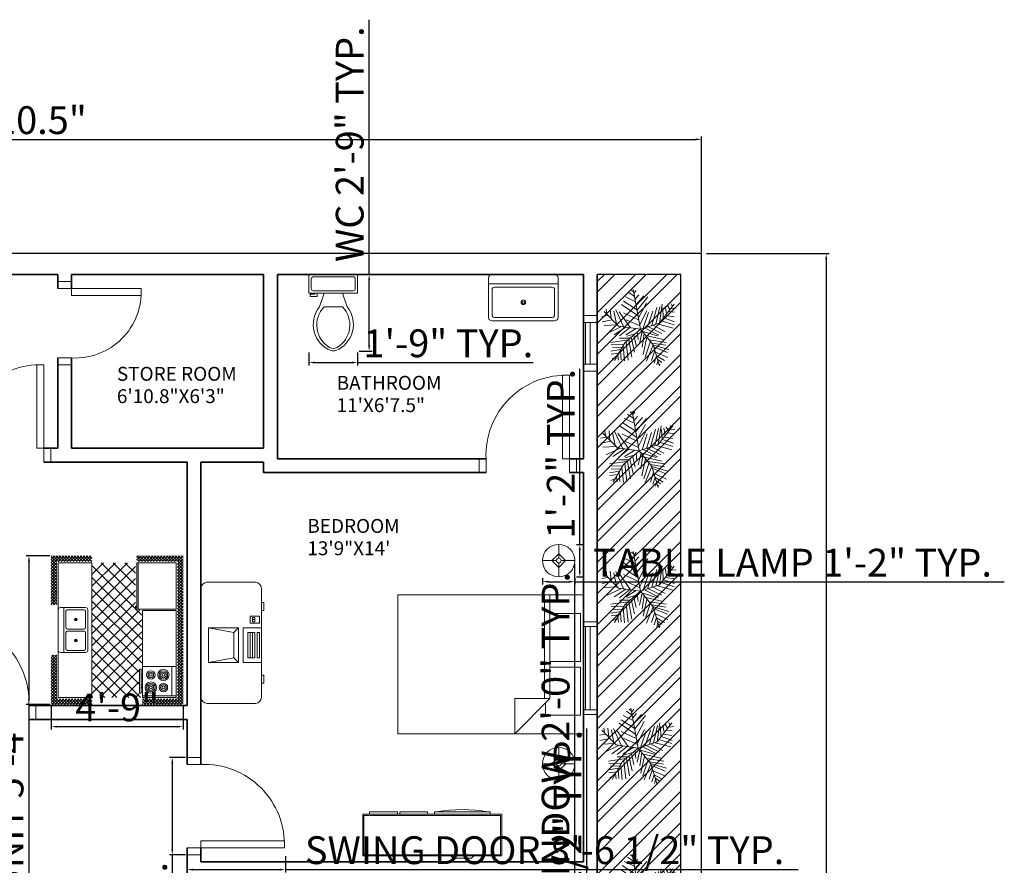
# Model space of a CAD drawing. Units: inches. Extents: x 2297 to 3143, y 440 to 1351.
# Tile 6 of 6: x 2697 to 3122, y 944 to 1309. Entities that reach past the tile are written whole.
import ezdxf

# ---------------------------------------------------------------- set-up
doc = ezdxf.new("R2010")
doc.units = ezdxf.units.IN
for name, color, linetype, lineweight in [('A-ANNO-DIMS', 2, 'Continuous', 18), ('A-AREA-IDEN', 7, 'Continuous', 18), ('A-DOOR', 4, 'Continuous', 20), ('A-EQPM', 8, 'Continuous', 18), ('A-FLOR-FIXT', 9, 'Continuous', 18), ('A-FURN', 8, 'Continuous', 18), ('A-GLAZ', 4, 'Continuous', 18), ('A-WALL', 7, 'Continuous', 35), ('C-PROP', 7, 'Continuous', 25), ('C-SITE-PATT', 252, 'Continuous', 13), ('E-LITE', 9, 'Continuous', 13), ('L-PLNT', 3, 'Continuous', 13)]:
    doc.layers.add(name, color=color, linetype=linetype, lineweight=lineweight)
doc.styles.get("Standard").update_dxf_attribs({"font": 'arial.ttf'})
doc.dimstyles.new('ISO-25', dxfattribs={"dimtxt": 12, "dimasz": 2.5, "dimexe": 1.25, "dimexo": 0.625, "dimtad": 1, "dimdec": 1, "dimlunit": 3, "dimtxsty": 'Standard', "dimcen": 2.5, "dimadec": 0, "dimazin": 0, "dimtfac": 1, "dimtdec": 1, "dimtmove": 0, "dimatfit": 3, "dimfxl": 1, "dimarcsym": 0})

# ---------------------------------------------------------------- blocks, each defined once
blk = doc.blocks.new('Kitchen Layout - 7 x 8 ft')
for p, q in [((-5, 81.32), (2.68, 89)), ((-5, 83.44), (0.56, 89)), ((-5, 85.56), (-1.56, 89)), ((-5, 87.68), (-3.68, 89)), ((-1, 84.97), (-5, 88.97)), ((-1, 82.85), (-5, 86.85)), ((-1, 80.73), (-5, 84.73)), ((1.09, 85), (-2.91, 89)), ((3.21, 85), (-0.79, 89)), ((0.81, 85), (4.81, 89)), ((5.34, 85), (1.34, 89)), ((2.93, 85), (6.93, 89)), ((7.46, 85), (3.46, 89)), ((5.05, 85), (9.05, 89)), ((9.58, 85), (5.58, 89)), ((7.17, 85), (11.17, 89)), ((11.7, 85), (7.7, 89)), ((9.29, 85), (13.29, 89)), ((13.82, 85), (9.82, 89)), ((11.41, 85), (15.41, 89)), ((15.94, 85), (11.94, 89)), ((13.53, 85), (17.53, 89)), ((18.06, 85), (14.06, 89)), ((15.65, 85), (19.65, 89)), ((20.18, 85), (16.18, 89)), ((17.78, 85), (21.78, 89)), ((22.31, 85), (18.31, 89)), ((19.9, 85), (23.9, 89)), ((24.43, 85), (20.43, 89)), ((22.02, 85), (26.02, 89)), ((26.55, 85), (22.55, 89)), ((24.14, 85), (28.14, 89)), ((28.67, 85), (24.67, 89)), ((26.26, 85), (30.26, 89)), ((30.79, 85), (26.79, 89)), ((28.38, 85), (32.38, 89)), ((32.91, 85), (28.91, 89)), ((30.5, 85), (34.5, 89)), ((35.03, 85), (31.03, 89)), ((32.63, 85), (36.63, 89)), ((37.16, 85), (33.16, 89)), ((34.75, 85), (38.75, 89)), ((39.28, 85), (35.28, 89)), ((36.87, 85), (40.87, 89)), ((41.4, 85), (37.4, 89)), ((38.99, 85), (42.99, 89)), ((43.52, 85), (39.52, 89)), ((41.11, 85), (45.11, 89)), ((45.64, 85), (41.64, 89)), ((43.23, 85), (47.23, 89)), ((47.76, 85), (43.76, 89)), ((45.35, 85), (49.35, 89)), ((49.88, 85), (45.88, 89)), ((47.47, 85), (51.47, 89)), ((52, 85), (48, 89)), ((49.6, 85), (53.6, 89)), ((54.13, 85), (50.13, 89)), ((51.72, 85), (55.72, 89)), ((56.25, 85), (52.25, 89)), ((53.84, 85), (57.84, 89)), ((58.37, 85), (54.37, 89)), ((55.96, 85), (59.96, 89)), ((60.49, 85), (56.49, 89)), ((58.08, 85), (62.08, 89)), ((62.61, 85), (58.61, 89)), ((60.2, 85), (64.2, 89)), ((64.73, 85), (60.73, 89)), ((62.32, 85), (66.32, 89)), ((66.85, 85), (62.85, 89)), ((64.45, 85), (68.45, 89)), ((68.97, 85), (64.97, 89)), ((66.57, 85), (70.57, 89)), ((71.1, 85), (67.1, 89)), ((68.69, 85), (72.69, 89)), ((73.22, 85), (69.22, 89)), ((70.81, 85), (74.81, 89)), ((75.34, 85), (71.34, 89)), ((72.93, 85), (76.93, 89)), ((77.46, 85), (73.46, 89)), ((75.05, 85), (79.05, 89)), ((79.58, 85), (75.58, 89)), ((77.17, 85), (81.17, 89)), ((81.7, 85), (77.7, 89)), ((79.29, 85), (83.29, 89)), ((83.82, 85), (79.82, 89)), ((81.42, 85), (85.42, 89)), ((85.95, 85), (81.95, 89)), ((83.54, 85), (87.54, 89)), ((88.07, 85), (84.07, 89)), ((85.66, 85), (89.66, 89)), ((90.19, 85), (86.19, 89)), ((87.78, 85), (91.78, 89)), ((92.31, 85), (88.31, 89)), ((89.9, 85), (93.9, 89)), ((94.43, 85), (90.43, 89)), ((92.02, 85), (96.02, 89)), ((96.55, 85), (92.55, 89)), ((94.14, 85), (98.14, 89)), ((101, 82.67), (94.67, 89)), ((96.27, 85), (100.27, 89)), ((101, 84.79), (96.79, 89)), ((97, 83.61), (101, 87.61)), ((97, 81.49), (101, 85.49)), ((101, 80.55), (97, 84.55)), ((101, 86.92), (98.92, 89)), ((-5, 79.19), (-1, 83.19)), ((-1, 78.61), (-5, 82.61)), ((-5, 77.07), (-1, 81.07)), ((-1, 76.49), (-5, 80.49)), ((-5, 74.95), (-1, 78.95)), ((-1, 74.36), (-5, 78.36)), ((34, 84), (96, 84)), ((34, 60), (34, 84)), ((74, 81), (95, 81)), ((96, 84), (96, 60)), ((97, 79.37), (101, 83.37)), ((101, 78.43), (97, 82.43)), ((97, 77.25), (101, 81.25)), ((101, 76.31), (97, 80.31)), ((97, 75.13), (101, 79.13)), ((101, 74.19), (97, 78.19)), ((-5, 72.83), (-1, 76.83)), ((-1, 72.24), (-5, 76.24)), ((-5, 70.71), (-1, 74.71)), ((-1, 70.12), (-5, 74.12)), ((-5, 68.59), (-1, 72.59)), ((-1, 68), (-5, 72)), ((-5, 66.47), (-1, 70.47)), ((97, 73.01), (101, 77.01)), ((101, 72.07), (97, 76.07)), ((97, 70.89), (101, 74.89)), ((101, 69.95), (97, 73.95)), ((97, 68.76), (101, 72.76)), ((101, 67.82), (97, 71.82)), ((97, 66.64), (101, 70.64)), ((-1, 65.88), (-5, 69.88)), ((-5, 64.35), (-1, 68.35)), ((-1, 63.76), (-5, 67.76)), ((-5, 62.22), (-1, 66.22)), ((-1, 61.64), (-5, 65.64)), ((-5, 60.1), (-1, 64.1)), ((-1, 59.52), (-5, 63.52)), ((101, 65.7), (97, 69.7)), ((97, 64.52), (101, 68.52)), ((101, 63.58), (97, 67.58)), ((97, 62.4), (101, 66.4)), ((101, 61.46), (97, 65.46)), ((97, 60.28), (101, 64.28)), ((100.34, 60), (97, 63.34)), ((-5, 57.98), (-1, 61.98)), ((-1, 57.39), (-5, 61.39)), ((-1.73, 56), (-5, 59.27)), ((-3.85, 56), (-5, 57.15)), ((-4.86, 56), (-1, 59.86)), ((-2.74, 56), (-1, 57.74)), ((0, 57), (33, 57)), ((10.4, 24), (45.9, 59.5)), ((18.88, 24), (54.38, 59.5)), ((27.37, 24), (62.87, 59.5)), ((33.03, 55.11), (37.41, 59.5)), ((67.71, 24), (33.68, 58.04)), ((96, 60), (34, 60)), ((35.85, 24), (71.35, 59.5)), ((76.2, 24), (40.7, 59.5)), ((44.34, 24), (77.84, 57.5)), ((84.68, 24), (49.18, 59.5)), ((52.82, 24), (86.32, 57.5)), ((93.17, 24), (57.67, 59.5)), ((61.31, 24), (96, 58.69)), ((96, 29.65), (66.15, 59.5)), ((96, 38.14), (76.64, 57.5)), ((80, 60), (80, 59)), ((82, 59), (82, 60)), ((96, 46.63), (85.13, 57.5)), ((87, 59), (87, 60)), ((89, 60), (89, 59)), ((96, 55.11), (93.57, 57.54)), ((98.22, 60), (97, 61.22)), ((98.84, 60), (101, 62.16)), ((100.96, 60), (101, 60.04)), ((0, 30.57), (24.43, 55)), ((0, 39.06), (15.94, 55)), ((0, 47.54), (7.46, 55)), ((25.29, 24), (0, 49.29)), ((1.91, 24), (32.91, 55)), ((33.77, 24), (2.77, 55)), ((42.26, 24), (11.26, 55)), ((50.74, 24), (19.74, 55)), ((59.23, 24), (28.23, 55)), ((31, 55), (31, 56)), ((32, 55), (31, 55)), ((32, 56), (32, 55)), ((69.79, 24), (96, 50.21)), ((16.8, 24), (0, 40.8)), ((78.28, 24), (96, 41.72)), ((8.32, 24), (0, 32.32)), ((86.76, 24), (96, 33.24)), ((-5, 21.92), (-2.92, 24)), ((-5, 19.8), (-1, 23.8)), ((-1, 19.21), (-5, 23.21)), ((-5, 17.68), (-1, 21.68)), ((-1, 17.09), (-5, 21.09)), ((-1, 21.33), (-3.67, 24)), ((-1, 23.45), (-1.55, 24)), ((0, 24), (96, 24)), ((0, 0), (0, 24)), ((95.25, 24), (96, 24.75)), ((96, 24), (96, 0)), ((97, 22.1), (98.9, 24)), ((97, 19.97), (101, 23.97)), ((101, 19.03), (97, 23.03)), ((97, 17.85), (101, 21.85)), ((101, 21.16), (98.16, 24)), ((101, 23.28), (100.28, 24)), ((-5, 15.55), (-1, 19.55)), ((-1, 14.97), (-5, 18.97)), ((-5, 13.43), (-1, 17.43)), ((-1, 12.85), (-5, 16.85)), ((-5, 11.31), (-1, 15.31)), ((-1, 10.73), (-5, 14.73)), ((47.25, 6.5), (47.25, 18.5)), ((48.75, 18.5), (48.75, 6.5)), ((101, 16.91), (97, 20.91)), ((97, 15.73), (101, 19.73)), ((101, 14.79), (97, 18.79)), ((97, 13.61), (101, 17.61)), ((101, 12.67), (97, 16.67)), ((97, 11.49), (101, 15.49)), ((101, 10.55), (97, 14.55)), ((-5, 9.19), (-1, 13.19)), ((-1, 8.6), (-5, 12.6)), ((-5, 7.07), (-1, 11.07)), ((-1, 6.48), (-5, 10.48)), ((-5, 4.95), (-1, 8.95)), ((-1, 4.36), (-5, 8.36)), ((97, 9.37), (101, 13.37)), ((101, 8.43), (97, 12.43)), ((97, 7.25), (101, 11.25)), ((101, 6.31), (97, 10.31)), ((97, 5.12), (101, 9.12)), ((101, 4.18), (97, 8.18)), ((-5, 2.83), (-1, 6.83)), ((-1, 2.24), (-5, 6.24)), ((-5, 0.71), (-1, 4.71)), ((-1, 0.12), (-5, 4.12)), ((-5, -1.42), (-1, 2.58)), ((2, -5), (-5, 2)), ((-5, -3.54), (-1, 0.46)), ((96, 0), (0, 0)), ((64, 4), (32, 4)), ((93.24, -5), (101, 2.76)), ((95.36, -5), (101, 0.64)), ((97, 3), (101, 7)), ((101, 2.06), (97, 6.06)), ((97, 0.88), (101, 4.88)), ((101, -0.06), (97, 3.94)), ((101, -2.18), (97, 1.82)), ((-0.12, -5), (-5, -0.12)), ((-2.25, -5), (-5, -2.25)), ((-4.37, -5), (-5, -4.37)), ((-4.34, -5), (-0.34, -1)), ((-2.22, -5), (1.78, -1)), ((-0.1, -5), (3.9, -1)), ((4.12, -5), (0.12, -1)), ((2.02, -5), (6.02, -1)), ((6.24, -5), (2.24, -1)), ((4.14, -5), (8.14, -1)), ((8.36, -5), (4.36, -1)), ((6.27, -5), (10.27, -1)), ((10.48, -5), (6.48, -1)), ((8.39, -5), (12.39, -1)), ((12.6, -5), (8.6, -1)), ((10.51, -5), (14.51, -1)), ((14.73, -5), (10.73, -1)), ((12.63, -5), (16.63, -1)), ((16.85, -5), (12.85, -1)), ((14.75, -5), (18.75, -1)), ((18.97, -5), (14.97, -1)), ((16.87, -5), (20.87, -1)), ((21.09, -5), (17.09, -1)), ((18.99, -5), (22.99, -1)), ((23.21, -5), (19.21, -1)), ((21.11, -5), (25.11, -1)), ((25.33, -5), (21.33, -1)), ((23.24, -5), (27.24, -1)), ((27.45, -5), (23.45, -1)), ((25.36, -5), (29.36, -1)), ((29.57, -5), (25.57, -1)), ((27.48, -5), (30, -2.48)), ((30, -3.3), (27.7, -1)), ((29.6, -5), (30, -4.6)), ((30, -1.18), (29.82, -1)), ((66, -2.54), (67.54, -1)), ((66, -4.66), (69.66, -1)), ((69.88, -5), (66, -1.12)), ((67.76, -5), (66, -3.24)), ((67.78, -5), (71.78, -1)), ((72, -5), (68, -1)), ((69.9, -5), (73.9, -1)), ((74.12, -5), (70.12, -1)), ((72.03, -5), (76.03, -1)), ((76.24, -5), (72.24, -1)), ((74.15, -5), (78.15, -1)), ((78.36, -5), (74.36, -1)), ((76.27, -5), (80.27, -1)), ((80.49, -5), (76.49, -1)), ((78.39, -5), (82.39, -1)), ((82.61, -5), (78.61, -1)), ((80.51, -5), (84.51, -1)), ((84.73, -5), (80.73, -1)), ((82.63, -5), (86.63, -1)), ((86.85, -5), (82.85, -1)), ((84.75, -5), (88.75, -1)), ((88.97, -5), (84.97, -1)), ((86.88, -5), (90.88, -1)), ((91.09, -5), (87.09, -1)), ((89, -5), (93, -1)), ((93.21, -5), (89.21, -1)), ((91.12, -5), (95.12, -1)), ((95.34, -5), (91.34, -1)), ((97.46, -5), (93.46, -1)), ((99.58, -5), (95.58, -1)), ((101, -4.3), (97, -0.3)), ((97.48, -5), (101, -1.48)), ((99.6, -5), (101, -3.6))]:
    blk.add_line(p, q)
for points in [[(0, 56), (0, 84), (33, 84), (33, 56)], [(74, 60), (74, 84), (95, 84), (95, 60)], [(76, 58), (76, 59), (93, 59), (93, 58)]]:
    blk.add_lwpolyline(points, close=True)
for points in [[(32, 1.5), (32, 19.5)], [(33.5, 21), (62.5, 21)], [(33.5, 6.5), (33.5, 18.5)], [(34.5, 19.5), (46.25, 19.5)], [(49.75, 19.5), (61.5, 19.5)], [(62.5, 18.5), (62.5, 6.5)], [(64, 19.5), (64, 1.5)], [(62.5, 0), (33.5, 0)], [(46.25, 5.5), (34.5, 5.5)], [(61.5, 5.5), (49.75, 5.5)]]:
    blk.add_lwpolyline(points)
for centre, radius in [((80, 75), 4), ((80, 75), 3), ((89, 75), 3), ((80, 75), 2), ((80, 75), 1), ((89, 75), 2), ((89, 75), 1), ((80, 66), 3), ((80, 66), 2), ((80, 66), 1), ((89, 66), 4), ((89, 66), 3), ((89, 66), 2), ((89, 66), 1), ((40.5, 12.5), 1), ((40.5, 12.5), 0.5), ((55.5, 12.5), 1), ((55.5, 12.5), 0.5)]:
    blk.add_circle(centre, radius)
for centre, radius, start, end in [((33.5, 19.5), 1.5, 90, 180), ((34.5, 18.5), 1, 90, 180), ((46.25, 18.5), 1, 0, 90), ((49.75, 18.5), 1, 90, 180), ((61.5, 18.5), 1, 0, 90), ((62.5, 19.5), 1.5, 0, 90), ((33.5, 1.5), 1.5, 180, 270), ((34.5, 6.5), 1, 180, 270), ((46.25, 6.5), 1, 270, 0), ((49.75, 6.5), 1, 180, 270), ((61.5, 6.5), 1, 270, 0), ((62.5, 1.5), 1.5, 270, 0)]:
    blk.add_arc(centre, radius, start, end)
blk = doc.blocks.new('Bed - Queen')
for p, q in [((0, -80.00003), (0, 0)), ((0, 0), (59.99999, 0)), ((59.99999, 0), (59.99999, -80.00003)), ((7.99999, -1.2), (28.79998, -1.2)), ((7.99999, -14.4), (7.99999, -1.2)), ((28.79998, -1.2), (28.79998, -14.4)), ((31.19999, -1.2), (51.99999, -1.2)), ((31.19999, -14.4), (31.19999, -1.2)), ((51.99999, -1.2), (51.99999, -16.4)), ((0, -14.4), (44.8, -14.4)), ((44.8, -16.8), (0, -16.8)), ((59.99999, -29.6), (44.8, -14.4)), ((44.8, -14.4), (44.8, -29.6)), ((51.99999, -16.4), (46.79936, -16.4)), ((44.8, -29.6), (59.99999, -29.6)), ((59.99999, -80.00003), (0, -80.00003))]:
    blk.add_line(p, q)
blk = doc.blocks.new('Sink-single - 30 in top')
blk.add_line((-15, -3.999996), (15, -3.999996))
for points in [[(-13.5, 0), (13.5, 0)], [(-15, -18.499996), (-15, -1.5)], [(15, -1.5), (15, -18.499996)], [(-13.5, -17.499996), (-13.5, -6.499996)], [(-12.5, -5.499996), (12.5, -5.499996)], [(13.5, -6.499996), (13.5, -17.499996)], [(13.5, -19.999996), (-13.5, -19.999996)], [(12.5, -18.499996), (-12.5, -18.499996)]]:
    blk.add_lwpolyline(points)
for radius in [1, 0.5]:
    blk.add_circle((0, -11.999996), radius)
for centre, radius, start, end in [((-13.5, -1.5), 1.5, 90, 180), ((13.5, -1.5), 1.5, 0, 90), ((-12.5, -6.499996), 1, 90, 180), ((12.5, -6.499996), 1, 0, 90), ((-13.5, -18.499996), 1.5, 180, 270), ((-12.5, -17.499996), 1, 180, 270), ((12.5, -17.499996), 1, 270, 0), ((13.5, -18.499996), 1.5, 270, 0)]:
    blk.add_arc(centre, radius, start, end)
blk = doc.blocks.new('Toilet - top')
for p, q in [((9.5, -6), (9.5, -2)), ((-8, -8.5), (-8, -8)), ((-7, -8), (-7, -9.5)), ((-4, -8), (-6, -14)), ((4, -8), (6, -14)), ((-10, -8.5), (-8, -8.5)), ((-10, -9.5), (-10, -8.5)), ((-7, -9.5), (-10, -9.5)), ((4, -14), (-4, -14))]:
    blk.add_line(p, q)
blk.add_lwpolyline([(10.5, -8), (10.5, 0), (-10.5, 0), (-10.5, -8)], close=True)
for points in [[(-9.5, -2), (-9.5, -6)], [(8.5, -1), (-8.5, -1)], [(-8.5, -7), (8.5, -7)]]:
    blk.add_lwpolyline(points)
for centre, radius, start, end in [((-8.62, -1.88), 0.884, 81.8699, 188.1301), ((8.62, -1.88), 0.884, 351.8699, 98.1301), ((-8.62, -6.12), 0.884, 171.8699, 278.1301), ((8.62, -6.12), 0.884, 261.8699, 8.1301), ((3.52, -21.58), 12.17, 141.4691, 247.9714), ((4.2, -21.82), 11.33, 136.3677, 238.9468), ((-3.52, -21.58), 12.17, 292.0284, 38.5307), ((-4.2, -21.82), 11.33, 301.053, 43.6321), ((0, -27.88), 4, 245.7318, 294.2682), ((0, -29), 4, 254.8605, 285.1395)]:
    blk.add_arc(centre, radius, start, end)
blk = doc.blocks.new('*U16')
for p, q in [((0, 0), (-10.5, 57)), ((-7.288, 39.707), (-21.778, 46.673)), ((-8.737, 47.138), (-17.069, 52.711)), ((-10.186, 53.64), (-13.084, 55.962)), ((-9.099, 51.782), (-6.563, 55.962)), ((-7.65, 43.423), (-2.578, 49.46)), ((-5.839, 35.992), (4.667, 48.067)), ((-5.114, 27.632), (10.463, 46.673)), ((-48.585, 21.131), (-49.309, 29.026)), ((-43.513, 28.561), (-42.427, 15.558)), ((-3.665, 19.273), (-27.574, 35.527)), ((-5.114, 28.097), (-24.676, 40.636)), ((-2.941, 16.486), (8.652, 37.85)), ((16.259, 5.805), (23.142, 31.348)), ((22.055, 7.198), (27.489, 32.277)), ((27, 9), (48, 36)), ((27.127, 9.056), (31.112, 35.992)), ((31.836, 30.883), (32.561, 16.486)), ((35.096, 32.741), (37.27, 22.524)), ((38.719, 34.134), (41.979, 28.561)), ((43.791, 29.954), (51.036, 30.883)), ((44.153, 36.456), (45.239, 32.741)), ((-47.498, 19.737), (-55.83, 18.344)), ((-31.5, 4.5), (-52.5, 25.5)), ((-38.442, 26.239), (-34.819, 7.663)), ((-35.544, 28.097), (-24.314, 3.947)), ((-14.533, 2.09), (-30.834, 25.31)), ((-24.314, 23.917), (-2.941, 13.7)), ((-1.129, 6.734), (9.014, 26.704)), ((3.942, 1.625), (11.187, 24.381)), ((10.101, 3.483), (17.708, 26.239)), ((33.285, 16.486), (48.862, 10.913)), ((36.183, 19.737), (48.137, 17.88)), ((40.53, 25.775), (48.862, 24.846)), ((-40.615, 13.7), (-55.105, 10.913)), ((-33.37, 6.269), (-52.207, 5.34)), ((-28.299, 3.483), (-47.86, -5.805)), ((-21.416, 3.018), (-38.079, -8.128)), ((0, 0), (-31.5, 4.5)), ((-15.982, 2.09), (-30.11, -9.521)), ((0, 0), (-22.5, -19.5)), ((-6.563, 1.161), (-21.416, -8.128)), ((-20.691, 13.7), (-1.129, 4.876)), ((0, 0), (27, 9)), ((0, 0), (18, -22.5)), ((6.478, 1.625), (26.04, -8.592)), ((11.187, 3.483), (30.749, -5.805)), ((18.07, 5.805), (35.096, -3.483)), ((24.229, 7.663), (46.688, 1.625)), ((29.662, 12.307), (48.137, 6.269)), ((-15.257, -12.772), (-30.11, -12.772)), ((-6.563, -5.805), (-19.967, -9.985)), ((-13.446, -11.378), (-8.737, -32.741)), ((-9.461, -8.592), (-6.201, -23.453)), ((-4.752, -3.483), (-3.665, -14.629)), ((2.493, -3.019), (-1.491, -20.202)), ((1.769, -2.555), (24.229, -9.521)), ((5.029, -6.27), (2.131, -25.775)), ((9.014, -11.378), (3.58, -35.992)), ((7.565, -9.056), (32.198, -14.629)), ((-17.431, -15.094), (-42.789, -18.809)), ((-24.314, -21.596), (-42.427, -22.06)), ((-26.849, -26.24), (-40.253, -25.775)), ((-22.5, -19.5), (-37.5, -45)), ((-25.038, -23.918), (-22.865, -45.281)), ((-20.691, -18.345), (-17.793, -44.352)), ((-17.069, -15.094), (-12.721, -40.172)), ((14.085, -16.951), (6.478, -40.172)), ((18.07, -22.524), (8.289, -45.745)), ((12.274, -15.094), (36.907, -18.809)), ((16.259, -19.738), (36.183, -22.989)), ((18, -22.5), (27, -52.5)), ((18.433, -22.524), (40.53, -29.026)), ((19.157, -25.311), (38.719, -33.206)), ((-28.299, -29.026), (-42.789, -31.348)), ((-30.834, -34.135), (-42.427, -35.528)), ((-34.457, -39.708), (-40.978, -42.494)), ((-32.646, -36.921), (-31.921, -44.352)), ((-29.023, -30.884), (-27.936, -43.887)), ((20.244, -30.419), (15.897, -44.816)), ((22.78, -37.85), (19.519, -48.532)), ((21.331, -32.741), (39.081, -40.636)), ((22.78, -38.314), (34.372, -44.816)), ((24.591, -45.745), (23.142, -50.854)), ((24.591, -43.423), (30.749, -47.603)), ((26.764, -49.925), (28.213, -50.854))]:
    blk.add_line(p, q)
blk = doc.blocks.new('*D17')
at = {"layer": 'A-ANNO-DIMS', "color": 0, "lineweight": -2, "transparency": 16777216}
for p, q in [((2393.19, 1208.26), (2393.19, 1258.2)), ((2991.69, 1208.26), (2991.69, 1258.2)), ((2395.69, 1256.95), (2989.19, 1256.95))]:
    blk.add_line(p, q, dxfattribs=at)
at = {"layer": 'A-ANNO-DIMS', "color": 0, "transparency": 16777216}
for points in [[(2395.69, 1257.36), (2395.69, 1256.53), (2393.19, 1256.95)], [(2989.19, 1257.36), (2989.19, 1256.53), (2991.69, 1256.95)]]:
    blk.add_solid(points, dxfattribs=at)
at = {"layer": 'Defpoints', "color": 0, "transparency": 16777216}
for p in [(2991.69, 1256.95), (2393.19, 1207.63), (2991.69, 1207.63)]:
    blk.add_point(p, dxfattribs=at)
at = {"layer": 'A-ANNO-DIMS', "color": 0, "transparency": 16777216, "insert": (2692.44, 1263.7), "char_height": 12, "attachment_point": 5}
blk.add_mtext('49\'-10.5"', dxfattribs=at)
blk = doc.blocks.new('*D18')
at = {"layer": 'A-ANNO-DIMS', "color": 0, "lineweight": -2, "transparency": 16777216}
for p, q in [((2993.8, 1207.63), (3046.74, 1207.63)), ((3045.49, 1205.13), (3045.49, 550.13)), ((2992.32, 547.63), (3046.74, 547.63))]:
    blk.add_line(p, q, dxfattribs=at)
at = {"layer": 'A-ANNO-DIMS', "color": 0, "transparency": 16777216}
for points in [[(3045.07, 1205.13), (3045.91, 1205.13), (3045.49, 1207.63)], [(3045.07, 550.13), (3045.91, 550.13), (3045.49, 547.63)]]:
    blk.add_solid(points, dxfattribs=at)
at = {"layer": 'Defpoints', "color": 0, "transparency": 16777216}
for p in [(2993.18, 1207.63), (2991.69, 547.63), (3045.49, 547.63)]:
    blk.add_point(p, dxfattribs=at)
at = {"layer": 'A-ANNO-DIMS', "color": 0, "transparency": 16777216, "insert": (3038.76, 877.63), "char_height": 12, "attachment_point": 5, "rotation": 90}
blk.add_mtext("55'", dxfattribs=at)
blk = doc.blocks.new('Lamp - Table')
for p, q in [((0, 7), (0, 1)), ((-1, 0), (-7, 0)), ((0, 3), (-3, 0)), ((-3, 0), (0, -3)), ((3, 0), (0, 3)), ((0, -3), (3, 0)), ((1, 0), (7, 0)), ((0, -1), (0, -7))]:
    blk.add_line(p, q)
for radius in [7, 1]:
    blk.add_circle((0, 0), radius)
blk = doc.blocks.new('Desk - 30 x 60 in.')
for p, q in [((-26.999995, 0), (26.999995, 0)), ((-29.999995, -27), (-29.999995, -3)), ((29.999995, -3), (29.999995, -27)), ((26.999995, -30), (-26.999995, -30)), ((-20.000005, -30), (-20.000005, -31)), ((-20.000005, -31), (-16.000005, -31)), ((-16.000005, -31), (-16.000005, -30)), ((15.999995, -31), (15.999995, -30)), ((19.999995, -31), (15.999995, -31)), ((19.999995, -30), (19.999995, -31))]:
    blk.add_line(p, q)
for centre, start, end in [((-26.499995, -3.5), 98.1301, 171.8699), ((26.499995, -3.5), 8.130102, 81.8699), ((-26.499995, -26.5), 188.1301, 261.8699), ((26.499995, -26.5), 278.1301, 351.8699)]:
    blk.add_arc(centre, 3.535534, start, end)
blk = doc.blocks.new('Computer Terminal')
for p, q in [((-10, 11.5), (5, 11.5)), ((-8, 0.5), (-10, 11.5)), ((-10, -1.5), (-10, 11.5)), ((5, 11.5), (3, 0.5)), ((5, 11.5), (5, -1.5)), ((-10, -1.5), (-8, 0.5)), ((3, 0.5), (-8, 0.5)), ((3, 0.5), (5, -1.5)), ((5, -1.5), (-10, -1.5)), ((-10, -11.5), (-10, -3.5)), ((-10, -3.5), (5, -3.5)), ((5, -3.5), (5, -11.5)), ((-8, -5.5), (-8, -8.5)), ((3, -5.5), (-8, -5.5)), ((3, -6.5), (-8, -6.5)), ((-8, -7.5), (3, -7.5)), ((3, -8.5), (3, -5.5)), ((10, -6.5), (7, -6.5)), ((7, -6.5), (7, -10.5)), ((9.5, -7.5), (7.5, -7.5)), ((7.5, -7.5), (7.5, -8.5)), ((8.5, -7.5), (8.5, -8.5)), ((9.5, -8.5), (9.5, -7.5)), ((10, -10.5), (10, -6.5)), ((5, -11.5), (-10, -11.5)), ((-8, -8.5), (3, -8.5)), ((-8, -9.5), (-8, -10.5)), ((3, -9.5), (-8, -9.5)), ((-8, -10.5), (3, -10.5)), ((3, -10.5), (3, -9.5)), ((7, -10.5), (10, -10.5)), ((7.5, -8.5), (9.5, -8.5))]:
    blk.add_line(p, q)
blk = doc.blocks.new('Entertainment Center')
for p, q in [((-4, 0), (-5, -1)), ((4, 0), (-4, 0)), ((5, -1), (4, 0)), ((-17, -19), (-17, -1)), ((-17, -1), (43, -1)), ((-16.5, -18.5), (-16.5, -1.5)), ((-16.5, -1.5), (42.5, -1.5)), ((42.5, -1.5), (42.5, -18.5)), ((43, -1), (43, -19)), ((43, -19), (-17, -19)), ((42.5, -18.5), (-16.5, -18.5)), ((-12, -20), (-12, -19)), ((12, -20), (-12, -20)), ((12, -19), (12, -20)), ((15, -20), (15, -19)), ((27, -20), (15, -20)), ((27, -19), (27, -20)), ((28, -20), (28, -19)), ((40, -20), (28, -20)), ((40, -19), (40, -20))]:
    blk.add_line(p, q)
blk.add_arc((0, 40), 61, 259.6111, 280.3889)
blk = doc.blocks.new('DOOR-36IN-6IN-JAMB')
for p, q in [((0, 6), (0, 0)), ((3, 6), (3, 0)), ((39, 6), (39, 0)), ((42, 6), (42, 0))]:
    blk.add_line(p, q)
blk.add_lwpolyline([(39, 6), (36, 6), (36, 42), (39, 42)], close=True)
blk.add_arc((37.5, 7.5), 34.53, 87.5104, 182.4896)
blk = doc.blocks.new('DOOR-30IN-LEAF')
blk.add_lwpolyline([(30, 0), (27, 0), (27, 30), (30, 30)], close=True)
blk.add_arc((28.5, 1.5), 28.54, 86.9872, 183.0128)
blk = doc.blocks.new('WIN-36IN-6IN-WALL')
for p, q in [((6, 40), (0, 40)), ((6, 38), (0, 38)), ((3, 38), (3, 2)), ((5, 38), (5, 2)), ((0, 2), (6, 2)), ((0, 0), (6, 0))]:
    blk.add_line(p, q)
blk = doc.blocks.new('WIN-18IN-6IN-WALL')
for p, q in [((6, 24), (0, 24)), ((6, 21), (0, 21)), ((1, 3), (1, 21)), ((3, 3), (3, 21)), ((0, 3), (6, 3)), ((0, 0), (6, 0))]:
    blk.add_line(p, q)
blk = doc.blocks.new('*D27')
at = {"layer": 'A-ANNO-DIMS', "color": 0, "lineweight": -2, "transparency": 16777216}
for p, q in [((2923.06, 1067.52), (2923.06, 1064.79)), ((2937.06, 1067.52), (2937.06, 1064.79)), ((2925.56, 1066.04), (2934.56, 1066.04)), ((2937.06, 1066.04), (3122.34, 1066.04))]:
    blk.add_line(p, q, dxfattribs=at)
at = {"layer": 'A-ANNO-DIMS', "color": 0, "transparency": 16777216}
for points in [[(2925.56, 1066.46), (2925.56, 1065.63), (2923.06, 1066.04)], [(2934.56, 1066.46), (2934.56, 1065.63), (2937.06, 1066.04)]]:
    blk.add_solid(points, dxfattribs=at)
at = {"layer": 'Defpoints', "color": 0, "transparency": 16777216}
for p in [(2923.06, 1068.14), (2937.06, 1068.14), (2937.06, 1066.04)]:
    blk.add_point(p, dxfattribs=at)
at = {"layer": 'A-ANNO-DIMS', "color": 0, "transparency": 16777216, "insert": (3030.95, 1072.7), "char_height": 12, "attachment_point": 5}
blk.add_mtext('TABLE LAMP 1\'-2" TYP.', dxfattribs=at)
blk = doc.blocks.new('*D28')
at = {"layer": 'A-ANNO-DIMS', "color": 0, "lineweight": -2, "transparency": 16777216}
for p, q in [((2939.16, 1082.14), (2939.16, 1157.91)), ((2937.69, 1082.14), (2940.41, 1082.14)), ((2939.16, 1070.64), (2939.16, 1079.64)), ((2937.69, 1068.14), (2940.41, 1068.14))]:
    blk.add_line(p, q, dxfattribs=at)
at = {"layer": 'A-ANNO-DIMS', "color": 0, "transparency": 16777216}
for points in [[(2938.75, 1079.64), (2939.58, 1079.64), (2939.16, 1082.14)], [(2938.75, 1070.64), (2939.58, 1070.64), (2939.16, 1068.14)]]:
    blk.add_solid(points, dxfattribs=at)
at = {"layer": 'Defpoints', "color": 0, "transparency": 16777216}
for p in [(2937.06, 1082.14), (2939.16, 1082.14), (2937.06, 1068.14)]:
    blk.add_point(p, dxfattribs=at)
at = {"layer": 'A-ANNO-DIMS', "color": 0, "transparency": 16777216, "insert": (2932.51, 1121.28), "char_height": 12, "attachment_point": 5, "rotation": 90}
blk.add_mtext('1\'-2" TYP.', dxfattribs=at)
blk = doc.blocks.new('*D29')
at = {"layer": 'A-ANNO-DIMS', "color": 0, "lineweight": -2, "transparency": 16777216}
for p, q in [((2769.69, 947.51), (2769.69, 940.52)), ((2812.11, 947.51), (2812.11, 940.52)), ((2772.19, 941.77), (2809.61, 941.77)), ((2812.11, 941.77), (3033.33, 941.77))]:
    blk.add_line(p, q, dxfattribs=at)
at = {"layer": 'A-ANNO-DIMS', "color": 0, "transparency": 16777216}
for points in [[(2772.19, 942.19), (2772.19, 941.35), (2769.69, 941.77)], [(2809.61, 942.19), (2809.61, 941.35), (2812.11, 941.77)]]:
    blk.add_solid(points, dxfattribs=at)
at = {"layer": 'Defpoints', "color": 0, "transparency": 16777216}
for p in [(2769.69, 948.13), (2812.11, 948.13), (2812.11, 941.77)]:
    blk.add_point(p, dxfattribs=at)
at = {"layer": 'A-ANNO-DIMS', "color": 0, "transparency": 16777216, "insert": (2923.97, 948.61), "char_height": 12, "attachment_point": 5}
blk.add_mtext('SWING DOOR 3\'-6 1/2" TYP.', dxfattribs=at)
blk = doc.blocks.new('*D30')
at = {"layer": 'A-ANNO-DIMS', "color": 0, "lineweight": -2, "transparency": 16777216}
for p, q in [((2769.07, 990.13), (2762.08, 990.13)), ((2763.33, 987.63), (2763.33, 950.63)), ((2769.07, 948.13), (2762.08, 948.13)), ((2763.33, 948.13), (2763.33, 871.25))]:
    blk.add_line(p, q, dxfattribs=at)
at = {"layer": 'A-ANNO-DIMS', "color": 0, "transparency": 16777216}
for points in [[(2762.91, 987.63), (2763.75, 987.63), (2763.33, 990.13)], [(2762.91, 950.63), (2763.75, 950.63), (2763.33, 948.13)]]:
    blk.add_solid(points, dxfattribs=at)
at = {"layer": 'Defpoints', "color": 0, "transparency": 16777216}
for p in [(2769.69, 990.13), (2763.33, 948.13), (2769.69, 948.13)]:
    blk.add_point(p, dxfattribs=at)
at = {"layer": 'A-ANNO-DIMS', "color": 0, "transparency": 16777216, "insert": (2756.57, 908.44), "char_height": 12, "attachment_point": 5, "rotation": 90}
blk.add_mtext('3\'-6" TYP.', dxfattribs=at)
blk = doc.blocks.new('*D43')
at = {"layer": 'A-ANNO-DIMS', "color": 0, "lineweight": -2, "transparency": 16777216}
for p, q in [((2937.09, 918.32), (2937.09, 1073.92)), ((2940.07, 918.32), (2935.84, 918.32)), ((2937.09, 896.82), (2937.09, 915.82)), ((2940.07, 894.32), (2935.84, 894.32))]:
    blk.add_line(p, q, dxfattribs=at)
at = {"layer": 'A-ANNO-DIMS', "color": 0, "transparency": 16777216}
for points in [[(2936.68, 915.82), (2937.51, 915.82), (2937.09, 918.32)], [(2936.68, 896.82), (2937.51, 896.82), (2937.09, 894.32)]]:
    blk.add_solid(points, dxfattribs=at)
at = {"layer": 'Defpoints', "color": 0, "transparency": 16777216}
for p in [(2937.09, 918.32), (2940.69, 918.32), (2940.69, 894.32)]:
    blk.add_point(p, dxfattribs=at)
at = {"layer": 'A-ANNO-DIMS', "color": 0, "transparency": 16777216, "insert": (2930.26, 997.37), "char_height": 12, "attachment_point": 5, "rotation": 90}
blk.add_mtext('WINDOW 2\'-0" TYP.', dxfattribs=at)
blk = doc.blocks.new('*D44')
at = {"layer": 'A-ANNO-DIMS', "color": 0, "lineweight": -2, "transparency": 16777216}
for p, q in [((2940.69, 918.95), (2940.69, 923.17)), ((2946.69, 918.95), (2946.69, 923.17)), ((2938.19, 921.92), (2935.69, 921.92)), ((2940.69, 921.92), (2946.69, 921.92)), ((2949.19, 921.92), (3026.09, 921.92))]:
    blk.add_line(p, q, dxfattribs=at)
at = {"layer": 'A-ANNO-DIMS', "color": 0, "transparency": 16777216}
for points in [[(2938.19, 922.34), (2938.19, 921.5), (2940.69, 921.92)], [(2949.19, 922.34), (2949.19, 921.5), (2946.69, 921.92)]]:
    blk.add_solid(points, dxfattribs=at)
at = {"layer": 'Defpoints', "color": 0, "transparency": 16777216}
for p in [(2940.69, 918.32), (2946.69, 921.92), (2946.69, 918.32)]:
    blk.add_point(p, dxfattribs=at)
at = {"layer": 'A-ANNO-DIMS', "color": 0, "transparency": 16777216, "insert": (2988.89, 928.67), "char_height": 12, "attachment_point": 5}
blk.add_mtext('0\'-6" TYP.', dxfattribs=at)
blk = doc.blocks.new('*D55')
at = {"layer": 'A-ANNO-DIMS', "color": 0, "lineweight": -2, "transparency": 16777216}
for p, q in [((2848.26, 1198.63), (2848.26, 1308.61)), ((2843.93, 1198.63), (2849.51, 1198.63)), ((2848.26, 1168.09), (2848.26, 1196.13)), ((2843.93, 1165.59), (2849.51, 1165.59))]:
    blk.add_line(p, q, dxfattribs=at)
at = {"layer": 'A-ANNO-DIMS', "color": 0, "transparency": 16777216}
for points in [[(2847.84, 1196.13), (2848.68, 1196.13), (2848.26, 1198.63)], [(2847.84, 1168.09), (2848.68, 1168.09), (2848.26, 1165.59)]]:
    blk.add_solid(points, dxfattribs=at)
at = {"layer": 'Defpoints', "color": 0, "transparency": 16777216}
for p in [(2843.3, 1198.63), (2848.26, 1198.63), (2843.3, 1165.59)]:
    blk.add_point(p, dxfattribs=at)
at = {"layer": 'A-ANNO-DIMS', "color": 0, "transparency": 16777216, "insert": (2841.43, 1254.87), "char_height": 12, "attachment_point": 5, "rotation": 90}
blk.add_mtext('WC 2\'-9" TYP.', dxfattribs=at)
blk = doc.blocks.new('*D56')
at = {"layer": 'A-ANNO-DIMS', "color": 0, "lineweight": -2, "transparency": 16777216}
for p, q in [((2822.3, 1164.96), (2822.3, 1159.38)), ((2843.3, 1164.96), (2843.3, 1159.38)), ((2824.8, 1160.63), (2840.8, 1160.63)), ((2843.3, 1160.63), (2919.07, 1160.63))]:
    blk.add_line(p, q, dxfattribs=at)
at = {"layer": 'A-ANNO-DIMS', "color": 0, "transparency": 16777216}
for points in [[(2824.8, 1161.05), (2824.8, 1160.21), (2822.3, 1160.63)], [(2840.8, 1161.05), (2840.8, 1160.21), (2843.3, 1160.63)]]:
    blk.add_solid(points, dxfattribs=at)
at = {"layer": 'Defpoints', "color": 0, "transparency": 16777216}
for p in [(2822.3, 1165.59), (2843.3, 1165.59), (2843.3, 1160.63)]:
    blk.add_point(p, dxfattribs=at)
at = {"layer": 'A-ANNO-DIMS', "color": 0, "transparency": 16777216, "insert": (2882.44, 1167.38), "char_height": 12, "attachment_point": 5}
blk.add_mtext('1\'-9" TYP.', dxfattribs=at)
blk = doc.blocks.new('*D58')
at = {"layer": 'A-ANNO-DIMS', "color": 0, "lineweight": -2, "transparency": 16777216}
for p, q in [((2942.26, 897.56), (2942.26, 1002.62)), ((2938.32, 897.56), (2943.51, 897.56)), ((2942.26, 869.63), (2942.26, 895.06)), ((2938.32, 867.13), (2943.51, 867.13))]:
    blk.add_line(p, q, dxfattribs=at)
at = {"layer": 'A-ANNO-DIMS', "color": 0, "transparency": 16777216}
for points in [[(2941.84, 895.06), (2942.67, 895.06), (2942.26, 897.56)], [(2941.84, 869.63), (2942.67, 869.63), (2942.26, 867.13)]]:
    blk.add_solid(points, dxfattribs=at)
at = {"layer": 'Defpoints', "color": 0, "transparency": 16777216}
for p in [(2937.69, 897.56), (2942.26, 897.56), (2937.69, 867.13)]:
    blk.add_point(p, dxfattribs=at)
at = {"layer": 'A-ANNO-DIMS', "color": 0, "transparency": 16777216, "insert": (2935.43, 951.34), "char_height": 12, "attachment_point": 5, "rotation": 90}
blk.add_mtext('2\'-6 1/2" TYP.', dxfattribs=at)
blk = doc.blocks.new('*D61')
at = {"layer": 'A-ANNO-DIMS', "color": 0, "lineweight": -2, "transparency": 16777216}
for p, q in [((2710.47, 1077.25), (2700.22, 1077.25)), ((2701.47, 1074.75), (2701.47, 1015.6)), ((2710.47, 1013.1), (2700.22, 1013.1)), ((2701.47, 1013.1), (2701.47, 855.98))]:
    blk.add_line(p, q, dxfattribs=at)
at = {"layer": 'A-ANNO-DIMS', "color": 0, "transparency": 16777216}
for points in [[(2701.05, 1074.75), (2701.89, 1074.75), (2701.47, 1077.25)], [(2701.05, 1015.6), (2701.89, 1015.6), (2701.47, 1013.1)]]:
    blk.add_solid(points, dxfattribs=at)
at = {"layer": 'Defpoints', "color": 0, "transparency": 16777216}
for p in [(2711.09, 1077.25), (2701.47, 1013.1), (2711.09, 1013.1)]:
    blk.add_point(p, dxfattribs=at)
at = {"layer": 'A-ANNO-DIMS', "color": 0, "transparency": 16777216, "insert": (2694.64, 933.29), "char_height": 12, "attachment_point": 5, "rotation": 90}
blk.add_mtext('KITCHEN UNIT 5\'-4"', dxfattribs=at)
blk = doc.blocks.new('*D62')
at = {"layer": 'A-ANNO-DIMS', "color": 0, "lineweight": -2, "transparency": 16777216}
for p, q in [((2711.09, 1012.47), (2711.09, 1002.23)), ((2767.98, 1012.47), (2767.98, 1002.23)), ((2713.59, 1003.48), (2765.48, 1003.48))]:
    blk.add_line(p, q, dxfattribs=at)
at = {"layer": 'A-ANNO-DIMS', "color": 0, "transparency": 16777216}
for points in [[(2713.59, 1003.89), (2713.59, 1003.06), (2711.09, 1003.48)], [(2765.48, 1003.89), (2765.48, 1003.06), (2767.98, 1003.48)]]:
    blk.add_solid(points, dxfattribs=at)
at = {"layer": 'Defpoints', "color": 0, "transparency": 16777216}
for p in [(2711.09, 1013.1), (2767.98, 1013.1), (2767.98, 1003.48)]:
    blk.add_point(p, dxfattribs=at)
at = {"layer": 'A-ANNO-DIMS', "color": 0, "transparency": 16777216, "insert": (2739.54, 1010.23), "char_height": 12, "attachment_point": 5}
blk.add_mtext('4\'-9"', dxfattribs=at)

msp = doc.modelspace()

# ---------------------------------------------------------------- hatches: boundary and pattern name
at = {"layer": 'C-SITE-PATT'}
h = msp.add_hatch(dxfattribs=at)
h.set_pattern_fill('ANSI32', color=256)
h.paths.add_polyline_path([(2438.19, 1198.63), (2402.19, 1198.63), (2402.19, 556.63), (2667.43, 556.63), (2742.43, 556.63), (2946.69, 556.63), (2982.69, 556.63), (2982.69, 1117.63), (2982.69, 1123.63), (2982.69, 1198.63), (2946.69, 1198.63), (2946.69, 1117.63), (2946.69, 700.63), (2806.19, 700.63), (2806.19, 580.63), (2738.57, 580.63), (2738.57, 589.63), (2735.57, 589.63), (2735.57, 625.63, 0.402069), (2702.6, 591.13, 0.401544), (2669.57, 625.63), (2669.57, 589.63), (2666.57, 589.63), (2666.57, 580.63), (2438.19, 580.63)])
h.paths.add_polyline_path([(2706.46, 558.2, -0.000472), (2706.46, 558.13, -0.000473)], flags=16)
h.paths.add_polyline_path([(2875.15, 576.11), (2920.92, 576.11), (2920.92, 585.31), (2875.15, 585.31)], flags=24)
h.paths.add_polyline_path([(2875.13, 585.74), (2915.96, 585.74), (2915.96, 595.05), (2875.13, 595.05)], flags=24)
h.paths.add_polyline_path([(2646.52, 1069.72), (2687.63, 1069.72), (2687.63, 1078.92), (2646.52, 1078.92)], flags=25)
h.paths.add_polyline_path([(2646.5, 1079.35), (2686.39, 1079.35), (2686.39, 1088.65), (2646.5, 1088.65)], flags=25)

# ---------------------------------------------------------------- linework, layer by layer
at = {"layer": 'A-DOOR'}
for p, q in [((2719.89, 1195.63), (2713.89, 1195.63)), ((2719.89, 1192.63), (2713.89, 1192.63)), ((2719.89, 1162.63), (2713.89, 1162.63)), ((2719.89, 1159.63), (2713.89, 1159.63))]:
    msp.add_line(p, q, dxfattribs=at)
at = {"layer": 'A-WALL'}
for p, q in [((2713.89, 1198.63), (2582.19, 1198.63)), ((2713.89, 1192.63), (2713.89, 1198.63)), ((2802.69, 1198.63), (2719.89, 1198.63)), ((2719.89, 1192.63), (2719.89, 1198.63)), ((2802.69, 1123.63), (2802.69, 1198.63)), ((2808.69, 1119.13), (2808.69, 1198.63)), ((2940.69, 1198.63), (2808.69, 1198.63)), ((2940.69, 1119.13), (2940.69, 1198.63)), ((2946.69, 1117.63), (2946.69, 1198.63)), ((2713.89, 1123.63), (2713.89, 1162.63)), ((2719.89, 1123.63), (2719.89, 1162.63)), ((2713.89, 1123.63), (2707.89, 1123.63)), ((2802.69, 1123.63), (2719.89, 1123.63)), ((2802.69, 1123.63), (2719.89, 1123.63)), ((2769.69, 1117.63), (2707.89, 1117.63)), ((2769.69, 1117.63), (2713.89, 1117.63)), ((2769.69, 1012.63), (2769.69, 1117.63)), ((2802.69, 1117.63), (2775.69, 1117.63)), ((2802.69, 1117.63), (2775.69, 1117.63)), ((2775.69, 987.13), (2775.69, 1117.63)), ((2802.69, 1113.13), (2802.69, 1117.63)), ((2898.69, 1119.13), (2808.69, 1119.13)), ((2940.69, 1119.13), (2934.69, 1119.13)), ((2946.69, 700.63), (2946.69, 1117.63)), ((2898.69, 1113.13), (2802.69, 1113.13)), ((2940.69, 1113.13), (2934.69, 1113.13)), ((2940.69, 945.13), (2940.69, 1113.13)), ((2769.69, 1012.63), (2701.46, 1012.63)), ((2769.69, 1006.63), (2701.46, 1006.63)), ((2769.69, 987.13), (2769.69, 1006.63)), ((2769.69, 939.13), (2769.69, 951.13)), ((2775.69, 945.13), (2775.69, 951.13)), ((2940.69, 945.13), (2775.69, 945.13))]:
    msp.add_line(p, q, dxfattribs=at)
at = {"layer": 'C-PROP'}
for p, q in [((2982.69, 1198.63), (2946.69, 1198.63)), ((2982.69, 1123.63), (2982.69, 1198.63)), ((2982.69, 1117.63), (2982.69, 1123.63)), ((2982.69, 556.63), (2982.69, 1117.63))]:
    msp.add_line(p, q, dxfattribs=at)
msp.add_lwpolyline([(2742.43, 547.63), (2991.69, 547.63), (2991.69, 1207.63), (2393.19, 1207.63)], dxfattribs=at)

# ---------------------------------------------------------------- block references
at = {"layer": 'A-DOOR', "extrusion": (0, 0, -1), "zscale": -1, "rotation": 89.99999999999999}
msp.add_blockref('DOOR-30IN-LEAF', (-2719.89, 1162.63), dxfattribs=at)
at = {"layer": 'A-DOOR'}
for p in [(2668.89, 1117.63), (2895.69, 1113.13)]:
    msp.add_blockref('DOOR-36IN-6IN-JAMB', p, dxfattribs=at)
at = {"layer": 'A-DOOR', "extrusion": (0, 0, -1), "zscale": -1}
msp.add_blockref('DOOR-36IN-6IN-JAMB', (-2704.46, 1006.63), dxfattribs=at)
at = {"layer": 'A-DOOR', "rotation": 269.999999999998}
msp.add_blockref('DOOR-36IN-6IN-JAMB', (2769.69, 990.13), dxfattribs=at)
at = {"layer": 'A-EQPM', "rotation": 89.99999999999999}
msp.add_blockref('Computer Terminal', (2790.38, 1041.16), dxfattribs=at)
at = {"layer": 'A-FLOR-FIXT'}
for name, p in [('Toilet - top', (2832.8, 1198.63)), ('Sink-single - 30 in top', (2914.79, 1198.63))]:
    msp.add_blockref(name, p, dxfattribs=at)
at = {"layer": 'A-FLOR-FIXT', "xscale": 0.605179280134624, "yscale": 0.605179280134624, "zscale": 0.605179280134624, "rotation": 270.0000000000005}
msp.add_blockref('Kitchen Layout - 7 x 8 ft', (2714.12, 1074.22), dxfattribs=at)
at = {"layer": 'A-FURN', "xscale": 0.8729228900222988, "yscale": 0.8729228900222988, "zscale": 0.8729228900222988, "rotation": 89.99999999999999}
msp.add_blockref('Desk - 30 x 60 in.', (2775.69, 1039.67), dxfattribs=at)
at = {"layer": 'A-FURN'}
for name, p, rotation in [('Bed - Queen', (2940.69, 1060.37), 270), ('Entertainment Center', (2888.48, 946.7), 180)]:
    msp.add_blockref(name, p, dxfattribs=dict(at, rotation=rotation))
at = {"layer": 'A-GLAZ'}
msp.add_blockref('WIN-18IN-6IN-WALL', (2940.69, 1156.91), dxfattribs=at)
at = {"layer": 'A-GLAZ', "rotation": 180}
msp.add_blockref('WIN-36IN-6IN-WALL', (2946.69, 1048.71), dxfattribs=at)
at = {"layer": 'E-LITE'}
for p in [(2930.06, 1075.14), (2930.07, 987.5)]:
    msp.add_blockref('Lamp - Table', p, dxfattribs=at)
at = {"layer": 'L-PLNT', "xscale": 0.3005060358918508, "yscale": 0.3005060358918508, "zscale": 0.3005060358918508}
for p in [(2965.39, 1174.97), (2964.85, 1122.52), (2965.39, 1061.95), (2964.38, 994.26), (2964.92, 931.29)]:
    msp.add_blockref('*U16', p, dxfattribs=at)

# ---------------------------------------------------------------- texts
at = {"layer": 'A-AREA-IDEN'}
for s, p in [('STORE ROOM', (2739.42, 1152.77)), ('BATHROOM', (2834.24, 1148.88)), ('6\'10.8"X6\'3"', (2739.42, 1143.13)), ('11\'X6\'7.5"', (2834.24, 1139.24)), ('BEDROOM', (2821.59, 1087.11)), ('13\'9"X14\'', (2821.59, 1077.48))]:
    msp.add_text(s, height=6, dxfattribs=at).set_placement(p)

# ---------------------------------------------------------------- dimensions: what is measured, and where the dimension line sits
at = {"layer": 'A-ANNO-DIMS'}
for base, p1, p2, angle, text, picture, middle in [((2848.26, 1198.63), (2843.3, 1165.59), (2843.3, 1198.63), 90, 'WC <> TYP.', '*D55', (2841.43, 1254.87)), ((2939.16, 1082.14), (2937.06, 1068.14), (2937.06, 1082.14), 90, '<> TYP.', '*D28', (2932.51, 1121.28)), ((2701.4701, 1013.0979), (2711.0925, 1077.2469), (2711.0925, 1013.0979), 270, 'KITCHEN UNIT <>', '*D61', (2694.6405, 933.2867)), ((2937.09, 918.32), (2940.69, 894.32), (2940.69, 918.32), 90, 'WINDOW <> TYP.', '*D43', (2930.26, 997.37)), ((2942.26, 897.56), (2937.69, 867.13), (2937.69, 897.56), 90, '<> TYP.', '*D58', (2935.43, 951.34)), ((2763.33, 948.13), (2769.69, 990.13), (2769.69, 948.13), 270, '<> TYP.', '*D30', (2756.57, 908.44))]:
    dim = msp.add_linear_dim(base=base, p1=p1, p2=p2, angle=angle, text=text, dimstyle='ISO-25', override={"dimdec": 1, "dimlfac": 1, "dimrnd": 0, "dimzin": 1, "dimdsep": 46, "dimlunit": 4, "dimfrac": 2}, dxfattribs=at)
    dim.commit()
    dim.dimension.update_dxf_attribs({"geometry": picture, "text_midpoint": middle})
dim = msp.add_linear_dim(base=(2991.69, 1256.95), p1=(2393.19, 1207.63), p2=(2991.69, 1207.63), dimstyle='ISO-25', override={"dimclrd": 0, "dimclre": 0, "dimclrt": 0}, dxfattribs=at)
dim.commit()
dim.dimension.update_dxf_attribs({"geometry": '*D17', "text_midpoint": (2692.44, 1263.7)})
for base, p1, p2, angle, override, picture, middle in [((3045.49, 547.63), (2993.18, 1207.63), (2991.69, 547.63), 90, {"dimclrd": 0, "dimclre": 0, "dimclrt": 0}, '*D18', (3038.76, 877.63)), ((2767.98, 1003.48), (2711.09, 1013.1), (2767.98, 1013.1), 0, {"dimdec": 1, "dimlfac": 1, "dimrnd": 0, "dimzin": 1, "dimdsep": 46, "dimlunit": 4, "dimfrac": 2}, '*D62', (2739.54, 1010.23))]:
    dim = msp.add_linear_dim(base=base, p1=p1, p2=p2, angle=angle, dimstyle='ISO-25', override=override, dxfattribs=at)
    dim.commit()
    dim.dimension.update_dxf_attribs({"geometry": picture, "text_midpoint": middle})
for base, p1, p2, text, picture, middle in [((2843.3, 1160.63), (2822.3, 1165.59), (2843.3, 1165.59), '<> TYP.', '*D56', (2882.44, 1167.38)), ((2937.06, 1066.04), (2923.06, 1068.14), (2937.06, 1068.14), 'TABLE LAMP <> TYP.', '*D27', (3030.95, 1072.7)), ((2812.11, 941.77), (2769.69, 948.13), (2812.11, 948.13), 'SWING DOOR <> TYP.', '*D29', (2923.97, 948.61)), ((2946.69, 921.92), (2940.69, 918.32), (2946.69, 918.32), '<> TYP.', '*D44', (2988.89, 928.67))]:
    dim = msp.add_linear_dim(base=base, p1=p1, p2=p2, text=text, dimstyle='ISO-25', override={"dimdec": 1, "dimlfac": 1, "dimrnd": 0, "dimzin": 1, "dimdsep": 46, "dimlunit": 4, "dimfrac": 2}, dxfattribs=at)
    dim.commit()
    dim.dimension.update_dxf_attribs({"geometry": picture, "text_midpoint": middle})

doc.saveas('drawing.dxf')
